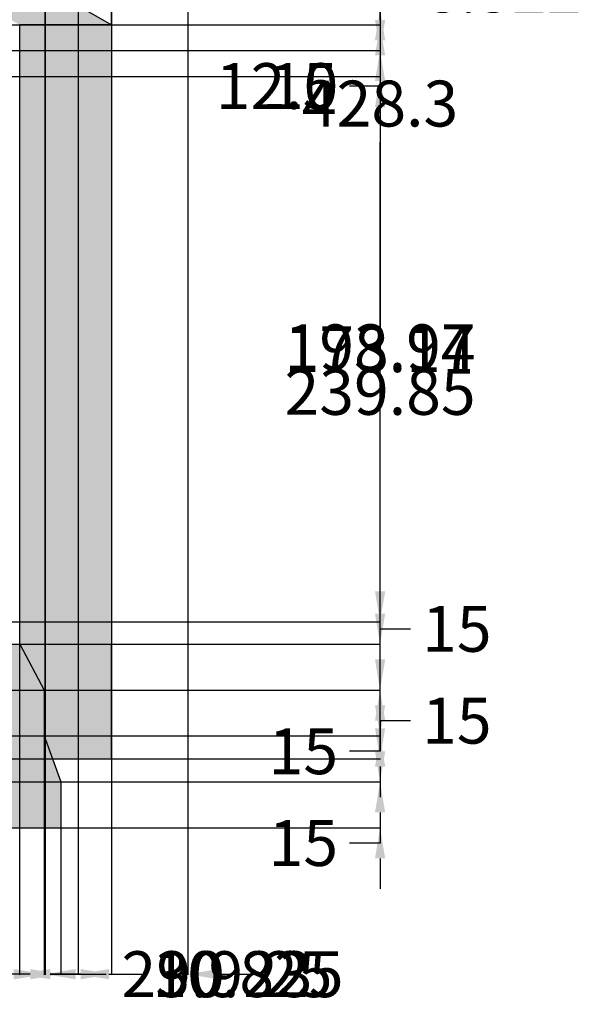
# Model space of a CAD drawing. Units: millimetres. Extents: x 131 to 845, y -20 to 1043.
# Tile 5 of 11: x 651 to 834, y -20 to 302. Entities that reach past the tile are written whole.
import ezdxf

# ---------------------------------------------------------------- set-up
doc = ezdxf.new("R2010")
doc.units = ezdxf.units.MM
doc.header["$MEASUREMENT"] = 0
for name, color, linetype, lineweight in [('A-ANNO-DIMS', 2, 'Continuous', 18), ('A-ELEV', 7, 'Continuous', 25), ('A-ELEV-PATT', 7, 'Continuous', 13), ('A-GLAZ-PATT', 143, 'Continuous', 13)]:
    doc.layers.add(name, color=color, linetype=linetype, lineweight=lineweight)
doc.styles.get("Standard").update_dxf_attribs({"font": 'arial.ttf'})
doc.dimstyles.get("Standard").update_dxf_attribs({"dimtxt": 15, "dimasz": 10, "dimexe": 0.18, "dimexo": 0.0625, "dimgap": 5, "dimtad": 0, "dimtih": 1, "dimtoh": 1, "dimdec": 0, "dimzin": 0, "dimdsep": 46, "dimtxsty": 'Standard', "dimcen": 5, "dimadec": 0, "dimazin": 0, "dimtfac": 1, "dimtdec": 0, "dimtofl": 0, "dimtmove": 0, "dimatfit": 3, "dimfxl": 1, "dimtolj": 1, "dimtzin": 0, "dimarcsym": 0})

# ---------------------------------------------------------------- blocks, each defined once
blk = doc.blocks.new('*D48')
at = {"layer": 'A-ANNO-DIMS', "color": 0, "lineweight": -2, "transparency": 16777216}
for p, q in [((680.53, 513.53), (680.53, -10.22)), ((705.53, 498.53), (705.53, -10.22)), ((670.53, -10.04), (660.53, -10.04)), ((715.53, -10.04), (725.53, -10.04))]:
    blk.add_line(p, q, dxfattribs=at)
at = {"layer": 'A-ANNO-DIMS', "color": 0, "transparency": 16777216}
for points in [[(670.53, -8.37), (670.53, -11.7), (680.53, -10.04)], [(715.53, -8.37), (715.53, -11.7), (705.53, -10.04)]]:
    blk.add_solid(points, dxfattribs=at)
at = {"layer": 'Defpoints', "color": 0, "transparency": 16777216}
for p in [(680.53, 513.6), (705.53, 498.6), (705.53, -10.04)]:
    blk.add_point(p, dxfattribs=at)
at = {"layer": 'A-ANNO-DIMS', "color": 0, "transparency": 16777216, "insert": (741.46, -10.04), "char_height": 15, "attachment_point": 5}
blk.add_mtext('\\A1;25', dxfattribs=at)
blk = doc.blocks.new('*D50')
at = {"layer": 'A-ANNO-DIMS', "color": 0, "lineweight": -2, "transparency": 16777216}
for p, q in [((720.6, 488.6), (768.56, 488.6)), ((768.38, 478.6), (768.38, 287.12)), ((768.38, 70.31), (768.38, 261.79)), ((216.3, 60.31), (768.56, 60.31))]:
    blk.add_line(p, q, dxfattribs=at)
at = {"layer": 'A-ANNO-DIMS', "color": 0, "transparency": 16777216}
for points in [[(766.72, 478.6), (770.05, 478.6), (768.38, 488.6)], [(766.72, 70.31), (770.05, 70.31), (768.38, 60.31)]]:
    blk.add_solid(points, dxfattribs=at)
at = {"layer": 'Defpoints', "color": 0, "transparency": 16777216}
for p in [(720.53, 488.6), (768.38, 488.6), (216.23, 60.31)]:
    blk.add_point(p, dxfattribs=at)
at = {"layer": 'A-ANNO-DIMS', "color": 0, "transparency": 16777216, "insert": (768.38, 274.45), "char_height": 15, "attachment_point": 5}
blk.add_mtext('\\A1;428.3', dxfattribs=at)
blk = doc.blocks.new('*D51')
at = {"layer": 'A-ANNO-DIMS', "color": 0, "lineweight": -2, "transparency": 16777216}
for p, q in [((658.81, 488.53), (658.81, -10.22)), ((628.88, 312.6), (628.88, -10.22)), ((618.88, -10.04), (608.88, -10.04)), ((668.81, -10.04), (678.81, -10.04))]:
    blk.add_line(p, q, dxfattribs=at)
at = {"layer": 'A-ANNO-DIMS', "color": 0, "transparency": 16777216}
for points in [[(618.88, -8.37), (618.88, -11.7), (628.88, -10.04)], [(668.81, -8.37), (668.81, -11.7), (658.81, -10.04)]]:
    blk.add_solid(points, dxfattribs=at)
at = {"layer": 'Defpoints', "color": 0, "transparency": 16777216}
for p in [(658.81, 488.6), (628.88, 312.66), (658.81, -10.04)]:
    blk.add_point(p, dxfattribs=at)
at = {"layer": 'A-ANNO-DIMS', "color": 0, "transparency": 16777216, "insert": (715.07, -10.04), "char_height": 15, "attachment_point": 5}
blk.add_mtext('\\A1;29.923', dxfattribs=at)
blk = doc.blocks.new('*D52')
at = {"layer": 'A-ANNO-DIMS', "color": 0, "lineweight": -2, "transparency": 16777216}
for p, q in [((669.71, 488.53), (669.71, -10.22)), ((658.88, 312.6), (658.88, -10.22)), ((648.88, -10.04), (638.88, -10.04)), ((679.71, -10.04), (689.71, -10.04))]:
    blk.add_line(p, q, dxfattribs=at)
at = {"layer": 'A-ANNO-DIMS', "color": 0, "transparency": 16777216}
for points in [[(648.88, -8.37), (648.88, -11.7), (658.88, -10.04)], [(679.71, -8.37), (679.71, -11.7), (669.71, -10.04)]]:
    blk.add_solid(points, dxfattribs=at)
at = {"layer": 'Defpoints', "color": 0, "transparency": 16777216}
for p in [(669.71, 488.6), (658.88, 312.66), (669.71, -10.04)]:
    blk.add_point(p, dxfattribs=at)
at = {"layer": 'A-ANNO-DIMS', "color": 0, "transparency": 16777216, "insert": (725.2, -10.04), "char_height": 15, "attachment_point": 5}
blk.add_mtext('\\A1;10.825', dxfattribs=at)
blk = doc.blocks.new('*D60')
at = {"layer": 'A-ANNO-DIMS', "color": 0, "lineweight": -2, "transparency": 16777216}
for p, q in [((768.38, 333.16), (768.38, 343.16)), ((768.38, 343.16), (778.38, 343.16)), ((617.11, 323.16), (768.56, 323.16)), ((617.11, 305.16), (768.56, 305.16)), ((768.38, 295.16), (768.38, 285.16))]:
    blk.add_line(p, q, dxfattribs=at)
at = {"layer": 'A-ANNO-DIMS', "color": 0, "transparency": 16777216}
for points in [[(766.72, 333.16), (770.05, 333.16), (768.38, 323.16)], [(766.72, 295.16), (770.05, 295.16), (768.38, 305.16)]]:
    blk.add_solid(points, dxfattribs=at)
at = {"layer": 'Defpoints', "color": 0, "transparency": 16777216}
for p in [(617.05, 323.16), (768.38, 323.16), (617.05, 305.16)]:
    blk.add_point(p, dxfattribs=at)
at = {"layer": 'A-ANNO-DIMS', "color": 0, "transparency": 16777216, "insert": (793.44, 343.16), "char_height": 15, "attachment_point": 5}
blk.add_mtext('\\A1;18', dxfattribs=at)
blk = doc.blocks.new('*D61')
at = {"layer": 'A-ANNO-DIMS', "color": 0, "lineweight": -2, "transparency": 16777216}
for p, q in [((768.38, 333.16), (768.38, 343.16)), ((768.38, 343.16), (778.38, 343.16)), ((617.11, 323.16), (768.56, 323.16)), ((617.11, 319.16), (768.56, 319.16)), ((768.38, 309.16), (768.38, 299.16))]:
    blk.add_line(p, q, dxfattribs=at)
at = {"layer": 'A-ANNO-DIMS', "color": 0, "transparency": 16777216}
for points in [[(766.72, 333.16), (770.05, 333.16), (768.38, 323.16)], [(766.72, 309.16), (770.05, 309.16), (768.38, 319.16)]]:
    blk.add_solid(points, dxfattribs=at)
at = {"layer": 'Defpoints', "color": 0, "transparency": 16777216}
for p in [(617.05, 323.16), (768.38, 323.16), (617.05, 319.16)]:
    blk.add_point(p, dxfattribs=at)
at = {"layer": 'A-ANNO-DIMS', "color": 0, "transparency": 16777216, "insert": (788.57, 343.16), "char_height": 15, "attachment_point": 5}
blk.add_mtext('\\A1;4', dxfattribs=at)
blk = doc.blocks.new('*D73')
at = {"layer": 'A-ANNO-DIMS', "color": 0, "lineweight": -2, "transparency": 16777216}
for p, q in [((650.53, 300.1), (650.53, -10.22)), ((680.53, 300.1), (680.53, -10.22)), ((660.53, -10.04), (670.53, -10.04)), ((680.53, -10.04), (690.53, -10.04))]:
    blk.add_line(p, q, dxfattribs=at)
at = {"layer": 'A-ANNO-DIMS', "color": 0, "transparency": 16777216}
for points in [[(660.53, -8.37), (660.53, -11.7), (650.53, -10.04)], [(670.53, -8.37), (670.53, -11.7), (680.53, -10.04)]]:
    blk.add_solid(points, dxfattribs=at)
at = {"layer": 'Defpoints', "color": 0, "transparency": 16777216}
for p in [(650.53, 300.16), (680.53, 300.16), (680.53, -10.04)]:
    blk.add_point(p, dxfattribs=at)
at = {"layer": 'A-ANNO-DIMS', "color": 0, "transparency": 16777216, "insert": (706.25, -10.04), "char_height": 15, "attachment_point": 5}
blk.add_mtext('\\A1;30', dxfattribs=at)
blk = doc.blocks.new('*D74')
at = {"layer": 'A-ANNO-DIMS', "color": 0, "lineweight": -2, "transparency": 16777216}
for p, q in [((680.6, 300.16), (768.56, 300.16)), ((768.38, 290.16), (768.38, 192.9)), ((768.38, 70.31), (768.38, 167.57)), ((680.6, 60.31), (768.56, 60.31))]:
    blk.add_line(p, q, dxfattribs=at)
at = {"layer": 'A-ANNO-DIMS', "color": 0, "transparency": 16777216}
for points in [[(766.72, 290.16), (770.05, 290.16), (768.38, 300.16)], [(766.72, 70.31), (770.05, 70.31), (768.38, 60.31)]]:
    blk.add_solid(points, dxfattribs=at)
at = {"layer": 'Defpoints', "color": 0, "transparency": 16777216}
for p in [(680.53, 300.16), (768.38, 300.16), (680.53, 60.31)]:
    blk.add_point(p, dxfattribs=at)
at = {"layer": 'A-ANNO-DIMS', "color": 0, "transparency": 16777216, "insert": (768.38, 180.24), "char_height": 15, "attachment_point": 5}
blk.add_mtext('\\A1;239.85', dxfattribs=at)
blk = doc.blocks.new('*D76')
at = {"layer": 'A-ANNO-DIMS', "color": 0, "lineweight": -2, "transparency": 16777216}
for p, q in [((768.38, 320.16), (768.38, 330.16)), ((472.3, 310.16), (768.56, 310.16)), ((489.62, 300.16), (768.56, 300.16)), ((768.38, 290.16), (768.38, 280.16)), ((768.38, 280.16), (758.38, 280.16))]:
    blk.add_line(p, q, dxfattribs=at)
at = {"layer": 'A-ANNO-DIMS', "color": 0, "transparency": 16777216}
for points in [[(766.72, 320.16), (770.05, 320.16), (768.38, 310.16)], [(766.72, 290.16), (770.05, 290.16), (768.38, 300.16)]]:
    blk.add_solid(points, dxfattribs=at)
at = {"layer": 'Defpoints', "color": 0, "transparency": 16777216}
for p in [(472.24, 310.16), (489.56, 300.16), (768.38, 300.16)]:
    blk.add_point(p, dxfattribs=at)
at = {"layer": 'A-ANNO-DIMS', "color": 0, "transparency": 16777216, "insert": (743.37, 280.16), "char_height": 15, "attachment_point": 5}
blk.add_mtext('\\A1;10', dxfattribs=at)
blk = doc.blocks.new('*D77')
at = {"layer": 'A-ANNO-DIMS', "color": 0, "lineweight": -2, "transparency": 16777216}
for p, q in [((648.88, 1033.52), (638.88, 1033.52)), ((658.88, 312.72), (658.88, 1033.7)), ((680.53, 300.22), (680.53, 1033.7)), ((690.53, 1033.52), (700.53, 1033.52))]:
    blk.add_line(p, q, dxfattribs=at)
at = {"layer": 'A-ANNO-DIMS', "color": 0, "transparency": 16777216}
for points in [[(648.88, 1035.18), (648.88, 1031.85), (658.88, 1033.52)], [(690.53, 1035.18), (690.53, 1031.85), (680.53, 1033.52)]]:
    blk.add_solid(points, dxfattribs=at)
at = {"layer": 'Defpoints', "color": 0, "transparency": 16777216}
for p in [(680.53, 1033.52), (658.88, 312.66), (680.53, 300.16)]:
    blk.add_point(p, dxfattribs=at)
at = {"layer": 'A-ANNO-DIMS', "color": 0, "transparency": 16777216, "insert": (731.03, 1033.52), "char_height": 15, "attachment_point": 5}
blk.add_mtext('\\A1;21.65', dxfattribs=at)
blk = doc.blocks.new('*D78')
at = {"layer": 'A-ANNO-DIMS', "color": 0, "lineweight": -2, "transparency": 16777216}
for p, q in [((768.38, 322.66), (768.38, 332.66)), ((658.95, 312.66), (768.56, 312.66)), ((680.6, 300.16), (768.56, 300.16)), ((768.38, 290.16), (768.38, 280.16)), ((768.38, 280.16), (758.38, 280.16))]:
    blk.add_line(p, q, dxfattribs=at)
at = {"layer": 'A-ANNO-DIMS', "color": 0, "transparency": 16777216}
for points in [[(766.72, 322.66), (770.05, 322.66), (768.38, 312.66)], [(766.72, 290.16), (770.05, 290.16), (768.38, 300.16)]]:
    blk.add_solid(points, dxfattribs=at)
at = {"layer": 'Defpoints', "color": 0, "transparency": 16777216}
for p in [(658.88, 312.66), (680.53, 300.16), (768.38, 300.16)]:
    blk.add_point(p, dxfattribs=at)
at = {"layer": 'A-ANNO-DIMS', "color": 0, "transparency": 16777216, "insert": (734.55, 280.16), "char_height": 15, "attachment_point": 5}
blk.add_mtext('\\A1;12.5', dxfattribs=at)
blk = doc.blocks.new('*D81')
at = {"layer": 'A-ANNO-DIMS', "color": 0, "lineweight": -2, "transparency": 16777216}
for p, q in [((498.97, 291.78), (768.56, 291.78)), ((768.38, 281.78), (768.38, 207.46)), ((768.38, 107.81), (768.38, 182.13)), ((498.97, 97.81), (768.56, 97.81))]:
    blk.add_line(p, q, dxfattribs=at)
at = {"layer": 'A-ANNO-DIMS', "color": 0, "transparency": 16777216}
for points in [[(766.72, 281.78), (770.05, 281.78), (768.38, 291.78)], [(766.72, 107.81), (770.05, 107.81), (768.38, 97.81)]]:
    blk.add_solid(points, dxfattribs=at)
at = {"layer": 'Defpoints', "color": 0, "transparency": 16777216}
for p in [(498.91, 291.78), (768.38, 291.78), (498.91, 97.81)]:
    blk.add_point(p, dxfattribs=at)
at = {"layer": 'A-ANNO-DIMS', "color": 0, "transparency": 16777216, "insert": (768.38, 194.8), "char_height": 15, "attachment_point": 5}
blk.add_mtext('\\A1;193.97', dxfattribs=at)
blk = doc.blocks.new('*D83')
at = {"layer": 'A-ANNO-DIMS', "color": 0, "lineweight": -2, "transparency": 16777216}
for p, q in [((602.06, 283.26), (768.56, 283.26)), ((768.38, 273.26), (768.38, 206.85)), ((768.38, 115.12), (768.38, 181.53)), ((602.06, 105.12), (768.56, 105.12))]:
    blk.add_line(p, q, dxfattribs=at)
at = {"layer": 'A-ANNO-DIMS', "color": 0, "transparency": 16777216}
for points in [[(766.72, 273.26), (770.05, 273.26), (768.38, 283.26)], [(766.72, 115.12), (770.05, 115.12), (768.38, 105.12)]]:
    blk.add_solid(points, dxfattribs=at)
at = {"layer": 'Defpoints', "color": 0, "transparency": 16777216}
for p in [(601.99, 283.26), (768.38, 283.26), (601.99, 105.12)]:
    blk.add_point(p, dxfattribs=at)
at = {"layer": 'A-ANNO-DIMS', "color": 0, "transparency": 16777216, "insert": (768.38, 194.19), "char_height": 15, "attachment_point": 5}
blk.add_mtext('\\A1;178.14', dxfattribs=at)
blk = doc.blocks.new('*D85')
at = {"layer": 'A-ANNO-DIMS', "color": 0, "lineweight": -2, "transparency": 16777216}
for p, q in [((768.38, 301.78), (768.38, 311.78)), ((768.38, 311.78), (778.38, 311.78)), ((639.93, 291.78), (768.56, 291.78)), ((602.06, 283.26), (768.56, 283.26)), ((768.38, 273.26), (768.38, 263.26))]:
    blk.add_line(p, q, dxfattribs=at)
at = {"layer": 'A-ANNO-DIMS', "color": 0, "transparency": 16777216}
for points in [[(766.72, 301.78), (770.05, 301.78), (768.38, 291.78)], [(766.72, 273.26), (770.05, 273.26), (768.38, 283.26)]]:
    blk.add_solid(points, dxfattribs=at)
at = {"layer": 'Defpoints', "color": 0, "transparency": 16777216}
for p in [(639.87, 291.78), (768.38, 291.78), (601.99, 283.26)]:
    blk.add_point(p, dxfattribs=at)
at = {"layer": 'A-ANNO-DIMS', "color": 0, "transparency": 16777216, "insert": (808.63, 311.78), "char_height": 15, "attachment_point": 5}
blk.add_mtext('\\A1;8.522', dxfattribs=at)
blk = doc.blocks.new('*D87')
at = {"layer": 'A-ANNO-DIMS', "color": 0, "lineweight": -2, "transparency": 16777216}
for p, q in [((768.38, 62.81), (768.38, 72.81)), ((768.38, 72.81), (778.38, 72.81)), ((664.04, 52.81), (768.56, 52.81)), ((664.04, 37.81), (768.56, 37.81)), ((768.38, 27.81), (768.38, 17.81))]:
    blk.add_line(p, q, dxfattribs=at)
at = {"layer": 'A-ANNO-DIMS', "color": 0, "transparency": 16777216}
for points in [[(766.72, 62.81), (770.05, 62.81), (768.38, 52.81)], [(766.72, 27.81), (770.05, 27.81), (768.38, 37.81)]]:
    blk.add_solid(points, dxfattribs=at)
at = {"layer": 'Defpoints', "color": 0, "transparency": 16777216}
for p in [(663.98, 52.81), (768.38, 52.81), (663.98, 37.81)]:
    blk.add_point(p, dxfattribs=at)
at = {"layer": 'A-ANNO-DIMS', "color": 0, "transparency": 16777216, "insert": (793.48, 72.81), "char_height": 15, "attachment_point": 5}
blk.add_mtext('\\A1;15', dxfattribs=at)
blk = doc.blocks.new('*D88')
at = {"layer": 'A-ANNO-DIMS', "color": 0, "lineweight": -2, "transparency": 16777216}
for p, q in [((768.38, 77.81), (768.38, 87.81)), ((658.58, 67.81), (768.56, 67.81)), ((664.04, 52.81), (768.56, 52.81)), ((768.38, 42.81), (768.38, 32.81)), ((768.38, 32.81), (758.38, 32.81))]:
    blk.add_line(p, q, dxfattribs=at)
at = {"layer": 'A-ANNO-DIMS', "color": 0, "transparency": 16777216}
for points in [[(766.72, 77.81), (770.05, 77.81), (768.38, 67.81)], [(766.72, 42.81), (770.05, 42.81), (768.38, 52.81)]]:
    blk.add_solid(points, dxfattribs=at)
at = {"layer": 'Defpoints', "color": 0, "transparency": 16777216}
for p in [(658.52, 67.81), (663.98, 52.81), (768.38, 52.81)]:
    blk.add_point(p, dxfattribs=at)
at = {"layer": 'A-ANNO-DIMS', "color": 0, "transparency": 16777216, "insert": (743.29, 32.81), "char_height": 15, "attachment_point": 5}
blk.add_mtext('\\A1;15', dxfattribs=at)
blk = doc.blocks.new('*D89')
at = {"layer": 'A-ANNO-DIMS', "color": 0, "lineweight": -2, "transparency": 16777216}
for p, q in [((768.38, 92.81), (768.38, 102.81)), ((768.38, 102.81), (778.38, 102.81)), ((658.58, 82.81), (768.56, 82.81)), ((658.58, 67.81), (768.56, 67.81)), ((768.38, 57.81), (768.38, 47.81))]:
    blk.add_line(p, q, dxfattribs=at)
at = {"layer": 'A-ANNO-DIMS', "color": 0, "transparency": 16777216}
for points in [[(766.72, 92.81), (770.05, 92.81), (768.38, 82.81)], [(766.72, 57.81), (770.05, 57.81), (768.38, 67.81)]]:
    blk.add_solid(points, dxfattribs=at)
at = {"layer": 'Defpoints', "color": 0, "transparency": 16777216}
for p in [(658.52, 82.81), (768.38, 82.81), (658.52, 67.81)]:
    blk.add_point(p, dxfattribs=at)
at = {"layer": 'A-ANNO-DIMS', "color": 0, "transparency": 16777216, "insert": (793.48, 102.81), "char_height": 15, "attachment_point": 5}
blk.add_mtext('\\A1;15', dxfattribs=at)
blk = doc.blocks.new('*D90')
at = {"layer": 'A-ANNO-DIMS', "color": 0, "lineweight": -2, "transparency": 16777216}
for p, q in [((768.38, 107.81), (768.38, 117.81)), ((650.6, 97.81), (768.56, 97.81)), ((658.58, 82.81), (768.56, 82.81)), ((768.38, 72.81), (768.38, 62.81)), ((768.38, 62.81), (758.38, 62.81))]:
    blk.add_line(p, q, dxfattribs=at)
at = {"layer": 'A-ANNO-DIMS', "color": 0, "transparency": 16777216}
for points in [[(766.72, 107.81), (770.05, 107.81), (768.38, 97.81)], [(766.72, 72.81), (770.05, 72.81), (768.38, 82.81)]]:
    blk.add_solid(points, dxfattribs=at)
at = {"layer": 'Defpoints', "color": 0, "transparency": 16777216}
for p in [(650.53, 97.81), (658.52, 82.81), (768.38, 82.81)]:
    blk.add_point(p, dxfattribs=at)
at = {"layer": 'A-ANNO-DIMS', "color": 0, "transparency": 16777216, "insert": (743.29, 62.81), "char_height": 15, "attachment_point": 5}
blk.add_mtext('\\A1;15', dxfattribs=at)
blk = doc.blocks.new('*D91')
at = {"layer": 'A-ANNO-DIMS', "color": 0, "lineweight": -2, "transparency": 16777216}
for p, q in [((459.56, 37.75), (459.56, -10.22)), ((663.98, 37.75), (663.98, -10.22)), ((469.56, -10.04), (531.36, -10.04)), ((653.98, -10.04), (592.17, -10.04))]:
    blk.add_line(p, q, dxfattribs=at)
at = {"layer": 'A-ANNO-DIMS', "color": 0, "transparency": 16777216}
for points in [[(469.56, -8.37), (469.56, -11.7), (459.56, -10.04)], [(653.98, -8.37), (653.98, -11.7), (663.98, -10.04)]]:
    blk.add_solid(points, dxfattribs=at)
at = {"layer": 'Defpoints', "color": 0, "transparency": 16777216}
for p in [(459.56, 37.81), (663.98, 37.81), (663.98, -10.04)]:
    blk.add_point(p, dxfattribs=at)
at = {"layer": 'A-ANNO-DIMS', "color": 0, "transparency": 16777216, "insert": (561.77, -10.04), "char_height": 15, "attachment_point": 5}
blk.add_mtext('\\A1;204.4', dxfattribs=at)
blk = doc.blocks.new('*D92')
at = {"layer": 'A-ANNO-DIMS', "color": 0, "lineweight": -2, "transparency": 16777216}
for p, q in [((459.56, 67.75), (459.56, -10.22)), ((658.52, 67.75), (658.52, -10.22)), ((469.56, -10.04), (523.62, -10.04)), ((648.52, -10.04), (594.46, -10.04))]:
    blk.add_line(p, q, dxfattribs=at)
at = {"layer": 'A-ANNO-DIMS', "color": 0, "transparency": 16777216}
for points in [[(469.56, -8.37), (469.56, -11.7), (459.56, -10.04)], [(648.52, -8.37), (648.52, -11.7), (658.52, -10.04)]]:
    blk.add_solid(points, dxfattribs=at)
at = {"layer": 'Defpoints', "color": 0, "transparency": 16777216}
for p in [(459.56, 67.81), (658.52, 67.81), (658.52, -10.04)]:
    blk.add_point(p, dxfattribs=at)
at = {"layer": 'A-ANNO-DIMS', "color": 0, "transparency": 16777216, "insert": (559.04, -10.04), "char_height": 15, "attachment_point": 5}
blk.add_mtext('\\A1;198.96', dxfattribs=at)

msp = doc.modelspace()

# ---------------------------------------------------------------- hatches: boundary and pattern name
at = {"layer": 'A-ELEV-PATT', "transparency": 33554681}
h = msp.add_hatch(color=256, dxfattribs=at)
h.set_gradient(color1=(79, 2, 22), color2=(153, 133, 76), name='SPHERICAL')
h.paths.add_polyline_path([(459.5586, 310.1596), (459.5586, 300.1596), (489.5586, 300.1596), (472.2381, 310.1596)])
h.paths.add_polyline_path([(658.8842, 312.6596), (628.8842, 312.6596), (650.5349, 300.1596), (680.5349, 300.1596)])
h = msp.add_hatch(color=256, dxfattribs=at)
h.set_gradient(color1=(255, 255, 255), color2=(199, 200, 202), name='INVSPHERICAL')
h.paths.add_polyline_path([(489.5586, 300.1596), (459.5586, 300.1596), (459.5586, 252.07), (459.5586, 97.8131), (489.5586, 97.8131)])
h.paths.add_polyline_path([(680.5349, 300.1596), (650.5349, 300.1596), (650.5349, 97.8131), (680.5349, 97.8131)])
h.paths.add_polyline_path([(658.5215, 82.8131), (459.5586, 82.8131), (459.5586, 67.8131), (658.5215, 67.8131)])
h.paths.add_polyline_path([(663.9762, 52.8131), (459.5586, 52.8131), (459.5586, 37.8131), (663.9762, 37.8131)])
h.paths.add_polyline_path([(680.5349, 97.8131), (650.5349, 97.8131), (658.5215, 82.8131), (658.5215, 67.8131), (661.2489, 60.3131), (680.5349, 60.3131)])
at = {"layer": 'A-GLAZ-PATT'}
h = msp.add_hatch(color=256, dxfattribs=at)
h.dxf.hatch_style = 1
h.paths.add_polyline_path([(658.8074, 488.5953), (628.8842, 488.5953), (628.8842, 312.6596), (658.8842, 312.6596)])
h.paths.add_polyline_path([(650.5349, 97.8131), (459.5586, 97.8131), (459.5586, 82.8131), (658.5215, 82.8131)])
h.paths.add_polyline_path([(658.5215, 67.8131), (459.5586, 67.8131), (459.5586, 52.8131), (663.9762, 52.8131)])

# ---------------------------------------------------------------- linework, layer by layer
at = {"layer": 'A-ELEV'}
for p, q in [((658.8842, 312.6596), (680.5349, 300.1596)), ((680.5349, 300.1596), (650.5349, 300.1596)), ((680.5349, 300.1596), (680.5349, 97.8131)), ((680.5349, 300.1596), (680.5349, 97.8131)), ((650.5349, 97.8131), (658.5215, 82.8131)), ((680.5349, 60.3131), (680.5349, 97.8131)), ((459.5586, 82.8131), (658.5215, 82.8131)), ((658.5215, 82.8131), (658.5215, 67.8131)), ((459.5586, 67.8131), (658.5215, 67.8131)), ((658.5215, 67.8131), (663.9762, 52.8131)), ((661.2489, 60.3131), (680.5349, 60.3131)), ((459.5586, 52.8131), (663.9762, 52.8131)), ((663.9762, 52.8131), (663.9762, 37.8131)), ((459.5586, 37.8131), (663.9762, 37.8131))]:
    msp.add_line(p, q, dxfattribs=at)

# ---------------------------------------------------------------- dimensions: what is measured, and where the dimension line sits
at = {"layer": 'A-ANNO-DIMS'}
for base, p1, p2, override, picture, middle in [((680.5349, 1033.5163), (658.8842, 312.6596), (680.5349, 300.1596), {"dimdec": 2, "dimlfac": 1, "dimrnd": 0, "dimzin": 0, "dimdsep": 46, "dimlunit": 2}, '*D77', (731.0277, 1033.5163)), ((705.5349, -10.0369), (680.5349, 513.5953), (705.5349, 498.5953), {"dimdec": 0, "dimlfac": 1, "dimrnd": 0, "dimzin": 0, "dimdsep": 46, "dimlunit": 2}, '*D48', (741.4626, -10.0369)), ((658.8074, -10.0369), (628.8842, 312.6596), (658.8074, 488.5953), {"dimdec": 3, "dimlfac": 1, "dimrnd": 0, "dimzin": 0, "dimdsep": 46, "dimlunit": 2}, '*D51', (715.0711, -10.0369)), ((669.7096, -10.0369), (658.8842, 312.6596), (669.7096, 488.5953), {"dimdec": 3, "dimlfac": 1, "dimrnd": 0, "dimzin": 0, "dimdsep": 46, "dimlunit": 2}, '*D52', (725.1956, -10.0369)), ((680.5349, -10.0369), (650.5349, 300.1596), (680.5349, 300.1596), {"dimdec": 0, "dimlfac": 1, "dimrnd": 0, "dimzin": 0, "dimdsep": 46, "dimlunit": 2}, '*D73', (706.2477, -10.0369)), ((658.5215, -10.0369), (459.5586, 67.8131), (658.5215, 67.8131), {"dimdec": 2, "dimlfac": 1, "dimrnd": 0, "dimzin": 0, "dimdsep": 46, "dimlunit": 2}, '*D92', (559.0401, -10.0369)), ((663.9762, -10.0369), (459.5586, 37.8131), (663.9762, 37.8131), {"dimdec": 1, "dimlfac": 1, "dimrnd": 0, "dimzin": 0, "dimdsep": 46, "dimlunit": 2}, '*D91', (561.7674, -10.0369))]:
    dim = msp.add_linear_dim(base=base, p1=p1, p2=p2, dimstyle='Standard', override=override, dxfattribs=at)
    dim.commit()
    dim.dimension.update_dxf_attribs({"geometry": picture, "text_midpoint": middle})
for base, p1, p2, override, picture, middle in [((768.3849, 488.5953), (216.2327, 60.3131), (720.5349, 488.5953), {"dimdec": 1, "dimlfac": 1, "dimrnd": 0, "dimzin": 0, "dimdsep": 46, "dimlunit": 2}, '*D50', (768.3849, 274.4542)), ((768.3849, 323.1596), (617.0467, 305.1596), (617.0467, 323.1596), {"dimdec": 0, "dimlfac": 1, "dimrnd": 0, "dimzin": 0, "dimdsep": 46, "dimlunit": 2}, '*D60', (793.4377, 343.1596)), ((768.3849, 323.1596), (617.0467, 319.1596), (617.0467, 323.1596), {"dimdec": 0, "dimlfac": 1, "dimrnd": 0, "dimzin": 0, "dimdsep": 46, "dimlunit": 2}, '*D61', (788.5725, 343.1596)), ((768.3849, 300.1596), (658.8842, 312.6596), (680.5349, 300.1596), {"dimdec": 1, "dimlfac": 1, "dimrnd": 0, "dimzin": 0, "dimdsep": 46, "dimlunit": 2}, '*D78', (734.553, 280.1596)), ((768.3849, 300.1596), (472.2381, 310.1596), (489.5586, 300.1596), {"dimdec": 0, "dimlfac": 1, "dimrnd": 0, "dimzin": 0, "dimdsep": 46, "dimlunit": 2}, '*D76', (743.3729, 280.1596)), ((768.3849, 291.7824), (601.9946, 283.2603), (639.8713, 291.7824), {"dimdec": 3, "dimlfac": 1, "dimrnd": 0, "dimzin": 0, "dimdsep": 46, "dimlunit": 2}, '*D85', (808.627, 311.7824)), ((768.3849, 300.1596), (680.5349, 60.3131), (680.5349, 300.1596), {"dimdec": 2, "dimlfac": 1, "dimrnd": 0, "dimzin": 0, "dimdsep": 46, "dimlunit": 2}, '*D74', (768.3849, 180.2363)), ((768.3849, 291.7824), (498.9074, 97.8131), (498.9074, 291.7824), {"dimdec": 2, "dimlfac": 1, "dimrnd": 0, "dimzin": 0, "dimdsep": 46, "dimlunit": 2}, '*D81', (768.3849, 194.7977)), ((768.3849, 283.2603), (601.9946, 105.1179), (601.9946, 283.2603), {"dimdec": 2, "dimlfac": 1, "dimrnd": 0, "dimzin": 0, "dimdsep": 46, "dimlunit": 2}, '*D83', (768.3849, 194.1891)), ((768.3849, 82.8131), (650.5349, 97.8131), (658.5215, 82.8131), {"dimdec": 0, "dimlfac": 1, "dimrnd": 0, "dimzin": 0, "dimdsep": 46, "dimlunit": 2}, '*D90', (743.2911, 62.8131)), ((768.3849, 82.8131), (658.5215, 67.8131), (658.5215, 82.8131), {"dimdec": 0, "dimlfac": 1, "dimrnd": 0, "dimzin": 0, "dimdsep": 46, "dimlunit": 2}, '*D89', (793.4787, 102.8131)), ((768.3849, 52.8131), (658.5215, 67.8131), (663.9762, 52.8131), {"dimdec": 0, "dimlfac": 1, "dimrnd": 0, "dimzin": 0, "dimdsep": 46, "dimlunit": 2}, '*D88', (743.2911, 32.8131)), ((768.3849, 52.8131), (663.9762, 37.8131), (663.9762, 52.8131), {"dimdec": 0, "dimlfac": 1, "dimrnd": 0, "dimzin": 0, "dimdsep": 46, "dimlunit": 2}, '*D87', (793.4787, 72.8131))]:
    dim = msp.add_linear_dim(base=base, p1=p1, p2=p2, angle=90, dimstyle='Standard', override=override, dxfattribs=at)
    dim.commit()
    dim.dimension.update_dxf_attribs({"geometry": picture, "text_midpoint": middle})

doc.saveas('drawing.dxf')
